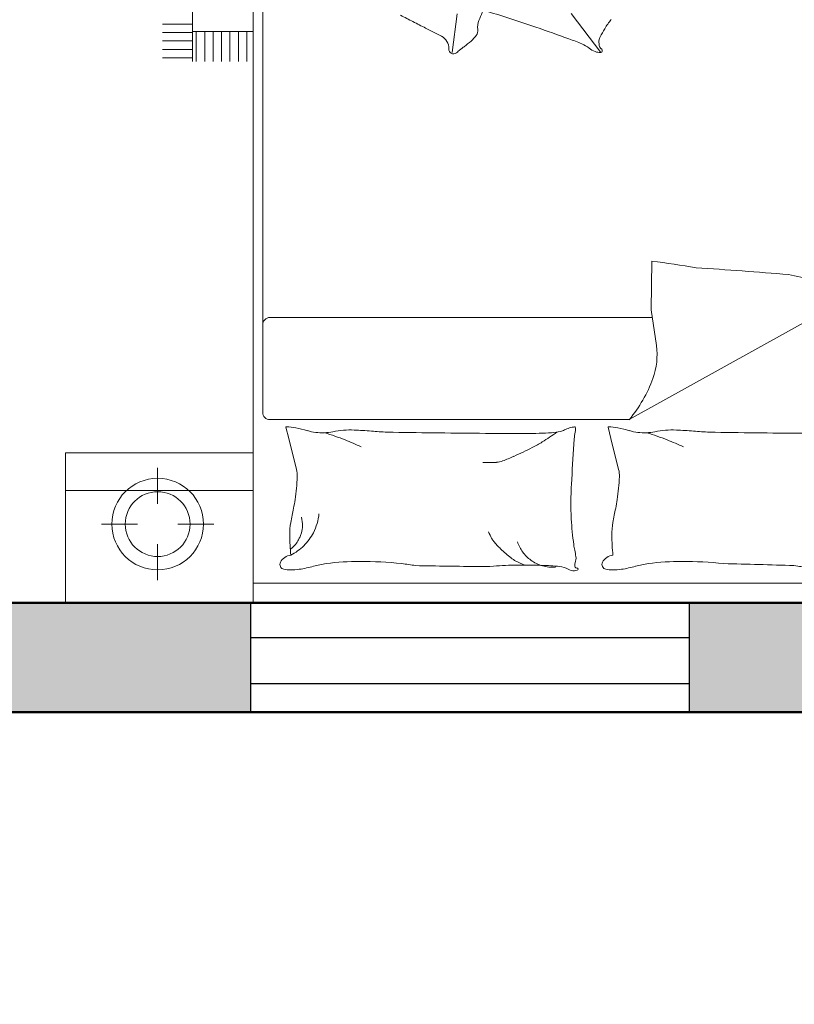
# Model space of a CAD drawing. Units: inches. Extents: x -7 to 1228, y -146 to 1091.
# Tile 36 of 88: x 1002 to 1066, y 36 to 117. Entities that reach past the tile are written whole.
import ezdxf

# ---------------------------------------------------------------- set-up
doc = ezdxf.new("R2010")
doc.units = ezdxf.units.IN
for name, color, linetype, lineweight in [('A-FURN', 8, 'Continuous', 18), ('A-GLAZ', 175, 'Continuous', 25), ('A-WALL', 7, 'Continuous', 50), ('A-WALL-PATT', 251, 'Continuous', 13)]:
    doc.layers.add(name, color=color, linetype=linetype, lineweight=lineweight)
doc.styles.add('DIM_FONT', font='SIMPLEX.shx', dxfattribs={"width": 0.8})

# ---------------------------------------------------------------- blocks, each defined once
blk = doc.blocks.new('A$C4F634EDD')
for p, q in [((0, 2.6295), (0, 2.2295)), ((0.5, 2.6295), (0, 2.6295)), ((0.5, 2.6295), (2.3, 2.6295)), ((0.5, 0.5295), (0.5, 2.6295)), ((0.5, 2.2295), (0.5, 2.6295)), ((0.5, 2.5771), (2.3, 2.5771)), ((0.2457, 2.5697), (0.2457, 2.4733)), ((0.0957, 2.4197), (0.192, 2.4197)), ((0.2994, 2.4197), (0.3957, 2.4197)), ((0.2457, 2.366), (0.2457, 2.2697)), ((0, 2.3301), (0.5, 2.3301)), ((0.5953, 2.1912), (0.616, 2.2738)), ((1.4546, 2.1912), (1.4752, 2.2738)), ((0, 2.2295), (0.5, 2.2295)), ((0.5878, 2.1612), (0.5953, 2.1912)), ((1.4471, 2.1612), (1.4546, 2.1912)), ((1.5035, 2.141), (0.5458, 2.141)), ((1.5035, 2.141), (2.2716, 1.7136)), ((0.5258, 2.121), (0.5258, 0.5617)), ((1.576, 1.9433), (1.5624, 1.8479)), ((0.5458, 1.8684), (1.5653, 1.8684)), ((1.5624, 1.8479), (1.5641, 1.7178)), ((0.3386, 0), (0.3386, 1.1852)), ((0.3486, 1.1052), (0.3486, 1.1852)), ((0.3711, 1.1052), (0.3711, 1.1852)), ((0.3936, 1.1052), (0.3936, 1.1852)), ((0.4161, 1.1052), (0.4161, 1.1852)), ((0.4386, 1.1052), (0.4386, 1.1852)), ((0.4611, 1.1052), (0.4611, 1.1852)), ((0.4836, 1.1052), (0.4836, 1.1852)), ((0.2586, 1.1753), (0.3386, 1.1753)), ((1.031, 1.1612), (1.0448, 1.0581)), ((1.4276, 1.1611), (1.3484, 1.0571)), ((0.2586, 1.1528), (0.3386, 1.1528)), ((0.2586, 1.1303), (0.3386, 1.1303)), ((0.2586, 1.1078), (0.3386, 1.1078)), ((0.3386, 1.1052), (0.5, 1.1052)), ((0.2586, 1.0853), (0.3386, 1.0853))]:
    blk.add_line(p, q)
for radius in [0.1222, 0.0865]:
    blk.add_circle((0.2457, 2.4197), radius)
for centre, radius, start, end in [((0.5848, 2.5274), 0.0131, 101.2724, 206.5805), ((0.5999, 2.4516), 0.0904, 90, 101.2724), ((0.5999, 2.3808), 0.1611, 81.5628, 90), ((0.5788, 2.2388), 0.3048, 74.256, 81.5628), ((0.7272, 2.7653), 0.2422, 254.256, 262.4531), ((0.7851, 3.2019), 0.6827, 262.4531, 270), ((0.7851, 3.5682), 1.049, 270, 276.0867), ((0.8402, 3.0514), 0.5293, 276.0867, 280.1899), ((1.1602, -8.1346), 10.6675, 90.30153, 91.21582), ((1.1169, 2.2433), 0.2897, 85.1982, 92.5386), ((1.2142, 3.4021), 0.8732, 265.1982, 269.4243), ((1.3082, 2.3102), 0.234, 110.8603, 117.2396), ((1.2204, 4.0232), 1.4943, 269.4243, 271.9079), ((1.2995, 2.4357), 0.0992, 105.9352, 126.0864), ((1.2429, 3.3501), 0.8208, 271.9079, 275.2592), ((1.2995, 2.4357), 0.0992, 85.7841, 105.9352), ((1.3132, 2.5864), 0.0539, 275.2592, 300.6513), ((1.3554, 2.5152), 0.0289, 85.6975, 120.6513), ((1.3556, 2.519), 0.0251, 68.2117, 85.6975), ((1.3739, 2.5288), 0.0156, 158.0096, 201.421), ((1.3634, 2.533), 0.00428, 78.1069, 158.0096), ((1.3288, 2.5111), 0.0328, 351.8665, 21.421), ((1.3647, 2.5395), 0.00232, 258.1069, 19.564), ((1.3637, 2.5391), 0.00342, 19.564, 68.2117), ((1.444, 2.5274), 0.0131, 101.2724, 206.5805), ((1.4591, 2.4516), 0.0904, 90, 101.2724), ((1.4591, 2.3808), 0.1611, 81.5628, 90), ((1.438, 2.2388), 0.3048, 74.256, 81.5628), ((1.5865, 2.7653), 0.2422, 254.256, 262.4531), ((1.6443, 3.2019), 0.6827, 262.4531, 270), ((1.6443, 3.5682), 1.049, 270, 276.0867), ((1.4785, 15.4878), 12.9656, 271.22425, 272.05324), ((1.97, 2.3805), 0.1524, 92.5386, 100.1899), ((0.6036, 2.5368), 0.0342, 206.5805, 265.5998), ((1.0898, 2.4496), 0.4918, 173.7676, 180), ((0.5368, 2.3783), 0.1399, 45.0976, 62.7964), ((1.4317, 2.2032), 0.3916, 128.3886, 133.8115), ((1.2362, 2.45), 0.0768, 117.2396, 128.3886), ((1.2995, 2.4357), 0.0992, 126.0864, 143.8234), ((1.1177, 2.5413), 0.246, 347.8905, 351.8665), ((1.4628, 2.5368), 0.0342, 206.5805, 265.5998), ((1.949, 2.4496), 0.4918, 173.7676, 180), ((0.5462, 2.4142), 0.0899, 41.4429, 53.7359), ((0.5741, 2.4389), 0.0526, 25.3551, 41.4429), ((0.5368, 2.3783), 0.1399, 27.3988, 45.0976), ((1.3165, 2.3233), 0.2252, 133.8115, 140.9651), ((1.2995, 2.4357), 0.0992, 143.8234, 161.5603), ((2.2605, 2.3525), 0.9131, 172.3191, 176.6313), ((1.5522, 2.448), 0.1983, 167.8905, 172.3191), ((0.8019, 2.4496), 0.204, 180, 189.6844), ((0.4851, 2.3967), 0.1511, 21.8149, 25.3551), ((0.4345, 2.3765), 0.2056, 18.7799, 21.8149), ((1.3127, 2.3625), 0.2002, 151.6832, 156.9972), ((1.1799, 2.4341), 0.0493, 140.9651, 151.6832), ((1.6611, 2.4496), 0.204, 180, 189.6844), ((0.576, 2.4246), 0.0562, 0, 18.7799), ((0.5406, 2.4246), 0.0915, 345.3149, 0), ((0.5368, 2.3783), 0.1399, 16.515, 27.3988), ((0.5368, 2.3783), 0.1399, 5.6311, 16.515), ((1.4703, 2.5637), 0.882, 189.6844, 192.1984), ((2.0266, 2.3663), 0.6787, 176.6313, 181.6331), ((2.3295, 2.5637), 0.882, 189.6844, 192.1984), ((0.2982, 2.3103), 0.3171, 8.0051, 12.1984), ((1.1575, 2.3103), 0.3171, 8.0051, 12.1984), ((-0.0401, 2.2627), 0.6588, 2.6649, 8.0051), ((2.7128, 2.3859), 1.3652, 181.6331, 183.055), ((0.8191, 2.2627), 0.6588, 2.6649, 8.0051), ((14.9657, 3.0398), 13.6356, 183.05496, 183.50486), ((0.5503, 2.2902), 0.0677, 345.9548, 2.6649), ((1.4096, 2.2902), 0.0677, 345.9548, 2.6649), ((1.1303, 1.9835), 0.2721, 85.9172, 93.5552), ((1.1455, 2.197), 0.058, 69.3257, 85.9172), ((0.9871, 1.7772), 0.5066, 65.6735, 69.3257), ((0.6058, 0.9338), 1.4323, 63.5015, 65.6735), ((0.473, 2.8815), 0.7387, 293.4844, 295.3111), ((1.1054, 1.9358), 0.3126, 57.865, 63.5015), ((1.3322, 2.8815), 0.7387, 293.4844, 295.3111), ((0.473, 2.8815), 0.7387, 287.1982, 289.428), ((0.473, 2.8815), 0.7387, 289.428, 291.6577), ((0.473, 2.8815), 0.7387, 291.6577, 293.4844), ((0.8841, 1.5835), 0.7286, 54.1737, 57.865), ((1.6762, 2.2258), 0.3212, 183.5049, 189.9984), ((1.3322, 2.8815), 0.7387, 287.1982, 289.428), ((1.3322, 2.8815), 0.7387, 289.428, 291.6577), ((1.3322, 2.8815), 0.7387, 291.6577, 293.4844), ((0.5887, 2.1609), 0.000917, 165.9551, 274.0829), ((0.5695, 2.4301), 0.2708, 274.0829, 279.4841), ((0.5763, 2.3896), 0.2297, 279.4841, 287.3864), ((0.6807, 2.0561), 0.1197, 96.4341, 107.3864), ((0.6836, 2.0301), 0.1459, 78.4414, 96.4341), ((0.759, 2.3985), 0.2301, 258.4414, 272.7491), ((0.7026, 3.5718), 1.4048, 272.7491, 274.6176), ((0.9136, 0.9591), 1.2165, 92.6096, 94.6176), ((1.2501, -19.8405), 22.0183, 90.37908, 91.01965), ((1.2012, -3.5404), 5.7185, 89.7135, 90.9704), ((1.224, 1.0141), 1.164, 86.426, 89.7135), ((1.2875, 2.0302), 0.1459, 77.131, 86.426), ((1.3099, 2.1283), 0.0453, 62.7159, 77.131), ((1.3658, 2.2367), 0.0767, 242.7159, 253.7788), ((1.3688, 2.247), 0.0875, 253.7788, 262.8796), ((1.3581, 2.1615), 0.00132, 262.8796, 343.3022), ((1.3409, 2.1667), 0.0193, 343.3022, 9.9984), ((1.448, 2.1609), 0.000917, 165.9551, 274.0829), ((1.4288, 2.4301), 0.2708, 274.0829, 279.4841), ((1.4355, 2.3896), 0.2297, 279.4841, 287.3864), ((1.5399, 2.0561), 0.1197, 96.4341, 107.3864), ((1.5429, 2.0301), 0.1459, 78.4414, 96.4341), ((1.6182, 2.3985), 0.2301, 258.4414, 272.7491), ((1.5619, 3.5718), 1.4048, 272.7491, 274.6176), ((1.7729, 0.9591), 1.2165, 92.6096, 94.6176), ((2.1093, -19.8405), 22.0183, 90.37908, 91.01965), ((0.5458, 2.121), 0.02, 90, 180), ((1.2147, 1.9017), 0.3751, 20.1488, 39.6445), ((1.3977, 1.9688), 0.1801, 351.8644, 20.1488), ((0.5458, 1.8884), 0.02, 180, 270), ((1.4194, 4.2174), 2.5158, 281.6741, 283.1904), ((1.0582, 5.4638), 3.7801, 277.692, 279.495), ((0.6102, 18.0525), 16.3521, 273.75703, 274.62393), ((1.0348, 1.1521), 0.0127, 51.1864, 183.2455), ((0.9991, 1.1077), 0.0697, 45.8726, 51.1864), ((1.0791, 1.1902), 0.0452, 225.8726, 232.4713), ((1.4338, 1.1026), 0.0601, 110.3452, 128.5854), ((1.4251, 1.1259), 0.0352, 86.0516, 110.3452), ((1.4273, 1.1567), 0.00443, 13.2808, 86.0516), ((1.4254, 1.1562), 0.0063, 306.5792, 13.2808), ((0.9863, 1.1494), 0.0359, 297.2902, 3.2455), ((1.2846, 1.4577), 0.3825, 232.4713, 233.7837), ((0.6683, 0.6162), 0.6605, 52.7849, 53.7837), ((0.9362, 0.9689), 0.2176, 46.4776, 52.7849), ((1.0543, 1.9106), 0.8371, 290.1287, 292.7069), ((1.3469, 1.2115), 0.0792, 292.7069, 308.5854), ((1.4996, 1.1284), 0.0771, 169.5926, 177.2714), ((1.4378, 1.1314), 0.0153, 177.2714, 194.5709), ((1.4376, 1.1398), 0.0142, 126.5792, 169.5926), ((-0.4173, 3.8699), 3.0972, 296.4147, 297.2902), ((1.0327, 1.0706), 0.0774, 35.8936, 46.4776), ((1.0771, 1.1027), 0.0226, 351.9508, 35.8936), ((-0.4107, 5.9078), 5.0942, 289.0836, 290.1287), ((1.4611, 1.1374), 0.0393, 194.5709, 206.8179), ((1.7401, 1.2785), 0.352, 206.8179, 210.9056), ((3.744, -4.3336), 6.1019, 117.49986, 117.84822), ((1.8575, -0.7096), 2.0162, 116.4147, 117.4999), ((1.1449, 1.0931), 0.0458, 171.9508, 202.4162), ((0.2266, 4.0657), 3.145, 286.6085, 289.0836), ((1.6045, 1.1973), 0.194, 210.9056, 219.7005), ((2.032, 1.4591), 1.0054, 202.4162, 205.0529)]:
    blk.add_arc(centre, radius, start, end)
at = {"style": 'DIM_FONT', "width": 0.8, "flags": 9}
for tag, p in [('YSIZE', (0.5, 2.6295)), ('XSIZE', (0.5, 2.6295)), ('XSIZE', (2.2985, 2.6295)), ('YSIZE', (2.2985, 2.6295))]:
    blk.add_attdef(tag, p, '', height=0.0005, dxfattribs=at)
blk = doc.blocks.new('WIN-36')
for p, q in [((0, 36), (0, 0)), ((9, 36), (0, 36)), ((2.343, 36), (2.343, 0)), ((6.137, 0), (6.137, 36)), ((9, 0), (9, 36)), ((0, 0), (9, 0)), ((2.343, 0), (6.137, 0))]:
    blk.add_line(p, q)

msp = doc.modelspace()

# ---------------------------------------------------------------- hatches: boundary and pattern name
at = {"layer": 'A-WALL-PATT'}
h = msp.add_hatch(color=256, dxfattribs=at)
h.dxf.hatch_style = 1
h.paths.add_polyline_path([(69, 568), (60, 568), (60, 493), (63.289, 493), (69, 493)])
h.paths.add_polyline_path([(69, 662.405), (60, 662.405), (60, 586), (69, 586)], flags=17)
h.paths.add_polyline_path([(69, 723), (184, 723), (184, 734), (179, 734), (179, 728), (69, 728), (69, 741.623), (60, 741.623), (60, 698.405), (69, 698.405)], flags=17)
h.paths.add_polyline_path([(69, 782), (231, 782), (231, 728), (231, 723), (231, 586), (236, 586), (236, 787), (69, 787), (69, 800.126), (60, 800.126), (60, 765.623), (69, 765.623)])
h.paths.add_polyline_path([(184, 842), (189, 842), (189, 848), (173, 848), (173, 842), (179, 842), (179, 787), (184, 787)])
h.paths.add_polyline_path([(118.22, 69), (69, 69), (69, 60), (118.22, 60)])
h.paths.add_polyline_path([(227, 69), (154.22, 69), (154.22, 60), (227, 60)])
h.paths.add_polyline_path([(236, 60), (232.711, 60), (227, 60), (227, 36), (236, 36)])
h.paths.add_polyline_path([(389, 60), (380, 60), (380, 36), (389, 36)])
h.paths.add_polyline_path([(384, 181), (380, 181), (380, 115), (380, 78), (384, 78)])
h.paths.add_polyline_path([(380, 115), (334.547, 115), (334.547, 109), (380, 109)])
h.paths.add_polyline_path([(274.547, 115), (236, 115), (236, 201), (232.711, 201), (231, 201), (231, 78), (236, 78), (236, 109), (274.547, 109)])
h.paths.add_polyline_path([(69, 123), (60, 123), (60, 78), (69, 78)])
h.paths.add_polyline_path([(69, 201), (60, 201), (60, 159), (69, 159)])
h.paths.add_polyline_path([(143, 219), (69, 219), (69, 213), (143, 213)], flags=17)
h.paths.add_polyline_path([(189, 219), (184, 219), (184, 274), (231, 274), (231, 219), (236, 219), (236, 279), (184, 279), (184, 297), (179, 297), (179, 279), (69, 279), (69, 290.912), (60, 290.912), (60, 262.179), (69, 262.179), (69, 274), (179, 274), (179, 219), (173, 219), (173, 213), (189, 213)])
h.paths.add_polyline_path([(69, 238.179), (60, 238.179), (60, 219), (69, 219)], flags=17)
h.paths.add_polyline_path([(69, 333), (60, 333), (60, 314.912), (69, 314.912), (69, 316.965)])
h.paths.add_polyline_path([(190, 338), (184, 338), (69, 338), (69, 333), (179, 333), (179, 327), (184, 327), (184, 333.021), (190, 333.046)])
h.paths.add_polyline_path([(69, 386.806), (60, 386.806), (60, 351), (69, 351)])
h.paths.add_polyline_path([(69, 475), (60, 475), (60, 422.806), (69, 422.806)])
h.paths.add_polyline_path([(236, 475), (231, 475), (231, 351.238), (236, 351.238)])
h.paths.add_polyline_path([(384, 475), (380, 475), (380, 362), (384, 362)])
h.paths.add_polyline_path([(547, 307), (439, 307), (439, 356), (445, 356), (445, 362), (433, 362), (433, 307), (380, 307), (380, 244), (380, 241), (384, 241), (384, 301), (433, 301), (433, 277), (439, 277), (439, 301), (547, 301)])
h.paths.add_polyline_path([(547, 241), (439, 241), (439, 247), (433, 247), (433, 235), (547, 235)])
h.paths.add_polyline_path([(450, 69), (440.286, 69), (424.889, 69), (389, 69), (389, 60), (450, 60)])
h.paths.add_polyline_path([(547, 69), (486, 69), (486, 60), (547, 60)])
h.paths.add_polyline_path([(556, 148.268), (547, 148.268), (547, 78), (556, 78)])
h.paths.add_polyline_path([(556, 223), (547, 223), (547, 195), (547, 184.268), (556, 184.268)])
h.paths.add_polyline_path([(556, 311.192), (547, 311.192), (547, 273.075), (556, 273.075)])
h.paths.add_polyline_path([(556, 344), (552.711, 344), (547, 344), (547, 335.192), (556, 335.192)])
h.paths.add_polyline_path([(556, 249.075), (547, 249.075), (547, 241), (556, 241)])
h.paths.add_polyline_path([(547, 362), (475, 362), (475, 356), (547, 356)], flags=0)
h.paths.add_polyline_path([(556, 399.621), (547, 399.621), (547, 362), (556, 362)])
h.paths.add_polyline_path([(556, 475), (547, 475), (547, 435.621), (556, 435.621)])
h.paths.add_polyline_path([(547, 493), (389, 493), (389, 487), (547, 487)])
h.paths.add_polyline_path([(380, 493), (278, 493), (278, 487), (380, 487)])
h.paths.add_polyline_path([(227, 493), (69, 493), (69, 487), (227, 487)])
h.paths.add_polyline_path([(643, 122.445), (634, 122.445), (634, 78), (643, 78)])
h.paths.add_polyline_path([(702.5, 69), (692.786, 69), (677.389, 69), (643, 69), (643, 60), (702.5, 60)])
h.paths.add_polyline_path([(798, 69), (738.5, 69), (738.5, 60), (798, 60)])
h.paths.add_polyline_path([(807, 60), (803.711, 60), (798, 60), (798, 36), (807, 36)])
h.paths.add_polyline_path([(807, 109), (846.751, 109), (846.751, 115), (807, 115), (807, 159), (802, 159), (802, 78), (807, 78)])
h.paths.add_polyline_path([(807, 201), (802, 201), (802, 195), (807, 195)])
h.paths.add_polyline_path([(643, 201), (634, 201), (634, 158.445), (643, 158.445)])
h.paths.add_polyline_path([(756, 225), (751, 225), (751, 219), (643, 219), (643, 213), (756, 213)])
h.paths.add_polyline_path([(643, 240.848), (634, 240.848), (634, 219), (643, 219)])
h.paths.add_polyline_path([(643, 274), (643, 288.629), (634, 288.629), (634, 264.848), (643, 264.848)])
h.paths.add_polyline_path([(802, 279), (756, 279), (756, 297), (751, 297), (751, 279), (643, 279), (643, 274), (751, 274), (751, 255), (756, 255), (756, 274), (802, 274)])
h.paths.add_polyline_path([(807, 333), (803.711, 333), (802, 333), (802, 279), (802, 274), (802, 219), (807, 219)])
h.paths.add_polyline_path([(956, 182), (951, 182), (951, 115), (906.751, 115), (906.751, 109), (951, 109), (951, 78), (956, 78)])
h.paths.add_polyline_path([(960, 60), (951, 60), (951, 36), (960, 36)])
h.paths.add_polyline_path([(1021, 69), (1005.781, 69), (960, 69), (960, 60), (1021, 60)])
h.paths.add_polyline_path([(956, 224), (951, 224), (951, 218), (956, 218)])
h.paths.add_polyline_path([(956, 302), (1004, 302), (1004, 278), (1010, 278), (1010, 302), (1118, 302), (1118, 290.809), (1127, 290.809), (1127, 326.968), (1118, 326.968), (1118, 320.966), (1118, 307), (1010, 307), (1010, 356), (1016, 356), (1016, 362), (1004, 362), (1004, 307), (951, 307), (951, 244), (951, 242), (954.289, 242), (956, 242)])
h.paths.add_polyline_path([(643, 333), (634, 333), (634, 312.629), (643, 312.629), (643, 316.965)])
h.paths.add_polyline_path([(756, 338), (643, 338), (643, 333), (751, 333), (751, 327), (756, 327)])
h.paths.add_polyline_path([(643, 388), (634, 388), (634, 351), (643, 351)])
h.paths.add_polyline_path([(807, 357), (802, 357), (802, 351), (807, 351)])
h.paths.add_polyline_path([(807, 475), (802, 475), (802, 393), (807, 393)])
h.paths.add_polyline_path([(643, 475), (634, 475), (634, 424), (643, 424)])
h.paths.add_polyline_path([(798, 493), (643, 493), (643, 487), (798, 487)])
h.paths.add_polyline_path([(634, 493), (556, 493), (556, 487), (634, 487)])
h.paths.add_polyline_path([(813, 493), (807, 493), (807, 487), (813, 487)])
h.paths.add_polyline_path([(951, 493), (849, 493), (849, 487), (951, 487)])
h.paths.add_polyline_path([(956, 484), (951, 484), (951, 374), (956, 374)])
h.paths.add_polyline_path([(1109, 493), (969, 493), (969, 487), (1109, 487)])
h.paths.add_polyline_path([(1127, 484), (1118, 484), (1118, 450.641), (1127, 450.641)])
h.paths.add_polyline_path([(1127, 414.641), (1118, 414.641), (1118, 365), (1127, 365)])
h.paths.add_polyline_path([(1109, 362), (1046, 362), (1046, 356), (1109, 356)], flags=17)
h.paths.add_polyline_path([(1127, 356), (1123.454, 356), (1118, 356), (1118, 350.968), (1127, 350.968)], flags=0)
h.paths.add_polyline_path([(1127, 266.809), (1118, 266.809), (1118, 262.361), (1118, 242), (1127, 242)], flags=17)
h.paths.add_polyline_path([(1118, 242), (1010, 242), (1010, 248), (1004, 248), (1004, 237), (1118, 237)])
h.paths.add_polyline_path([(1127, 224), (1118, 224), (1118, 170), (1127, 170)])
h.paths.add_polyline_path([(1127, 134), (1118, 134), (1118, 78), (1127, 78)])
h.paths.add_polyline_path([(1118, 69), (1057, 69), (1057, 60), (1118, 60)])
h.paths.add_polyline_path([(227, 571.546), (227, 574), (69, 574), (69, 568), (227, 568)])
h.paths.add_polyline_path([(380, 571.546), (380, 574), (278, 574), (278, 568), (380, 568)])
h.paths.add_polyline_path([(242, 574), (236, 574), (236, 568), (242, 568)])
h.paths.add_polyline_path([(547, 571.546), (547, 574), (389, 574), (389, 568), (547, 568)])
h.paths.add_polyline_path([(384, 733), (380, 733), (380, 586), (384, 586)])
h.paths.add_polyline_path([(556, 646), (634, 646), (634, 655), (547, 655), (547, 586), (556, 586)])
h.paths.add_polyline_path([(634, 574), (556, 574), (556, 568), (634, 568)])
h.paths.add_polyline_path([(643, 655), (634, 655), (634, 586), (643, 586)])
h.paths.add_polyline_path([(798, 574), (643, 574), (643, 568), (798, 568)])
h.paths.add_polyline_path([(643, 663.854), (634, 663.854), (634, 655), (643, 655)])
h.paths.add_polyline_path([(556, 676.967), (547, 676.967), (547, 655), (556, 655)])
h.paths.add_polyline_path([(556, 733), (547, 733), (547, 712.967), (556, 712.967)])
h.paths.add_polyline_path([(643, 710), (634, 710), (634, 699.854), (643, 699.854)])
h.paths.add_polyline_path([(807, 668), (802, 668), (802, 586), (807, 586)])
h.paths.add_polyline_path([(951, 574), (849, 574), (849, 568), (951, 568)])
h.paths.add_polyline_path([(956, 691), (951, 691), (951, 577), (956, 577)])
h.paths.add_polyline_path([(1109, 574), (969, 574), (969, 568), (1109, 568)])
h.paths.add_polyline_path([(1127, 643.403), (1118, 643.403), (1118, 577), (1127, 577)])
h.paths.add_polyline_path([(1127, 568), (1123.454, 568), (1118, 568), (1118, 493), (1127, 493)])
h.paths.add_polyline_path([(1127, 733), (1118, 733), (1118, 679.403), (1127, 679.403)])
h.paths.add_polyline_path([(1127, 777.348), (1118, 777.348), (1118, 770.035), (1118, 751), (1127, 751)], flags=17)
h.paths.add_polyline_path([(1118, 751), (1010, 751), (1010, 757), (1004, 757), (1004, 745), (1118, 745)])
h.paths.add_polyline_path([(956, 811), (1004, 811), (1004, 787), (1010, 787), (1010, 811), (1017.874, 811), (1017.874, 811.627, -0.414214), (1018.247, 812), (1031.978, 812, -0.414214), (1032.351, 811.627), (1032.351, 811), (1118, 811), (1118, 801.348), (1127, 801.348), (1127, 834.685), (1118, 834.685), (1118, 830.238), (1118, 817), (1010, 817), (1010, 866), (1016, 866), (1016, 872), (1004, 872), (1004, 817), (956, 817), (956, 866), (951, 866), (951, 751), (954.289, 751), (956, 751)])
h.paths.add_polyline_path([(1118, 872), (1046, 872), (1046, 866), (1118, 866)], flags=17)
h.paths.add_polyline_path([(1127, 924.711), (1118, 924.711), (1118, 884), (1127, 884)])
h.paths.add_polyline_path([(1127, 866), (1123.711, 866), (1118, 866), (1118, 858.685), (1127, 858.685)], flags=17)
h.paths.add_polyline_path([(956, 983), (951, 983), (951, 952), (807, 952), (807, 983), (802, 983), (802, 902), (807, 902), (807, 946), (951, 946), (951, 884), (956, 884)])
h.paths.add_polyline_path([(807, 842), (802, 842), (802, 787), (756, 787), (756, 806), (751, 806), (751, 787), (643, 787), (643, 782), (751, 782), (751, 764), (756, 764), (756, 782), (802, 782), (802, 728), (807, 728)])
h.paths.add_polyline_path([(756, 848), (643, 848), (643, 842), (751, 842), (751, 836), (756, 836)])
h.paths.add_polyline_path([(756, 734), (751, 734), (751, 728), (643, 728), (643, 723), (756, 723)])
h.paths.add_polyline_path([(643, 749.791), (634, 749.791), (634, 728), (637.289, 728), (643, 728)])
h.paths.add_polyline_path([(643, 805.405), (634, 805.405), (634, 773.791), (643, 773.791)])
h.paths.add_polyline_path([(643, 896.663), (634, 896.663), (634, 860), (637.289, 860), (643, 860)])
h.paths.add_polyline_path([(643, 842), (634, 842), (634, 829.405), (643, 829.405)])
h.paths.add_polyline_path([(643, 983), (634, 983), (634, 932.663), (643, 932.663)])
h.paths.add_polyline_path([(1127, 983), (1118, 983), (1118, 960.711), (1127, 960.711)])
h.paths.add_polyline_path([(1118, 1001), (1077.525, 1001), (1077.525, 992), (1118, 992)])
h.paths.add_polyline_path([(1041.525, 1001), (960, 1001), (960, 992), (1041.525, 992)])
h.paths.add_polyline_path([(960, 1025), (951, 1025), (951, 1001), (954.289, 1001), (960, 1001)])
h.paths.add_polyline_path([(807, 1025), (798, 1025), (798, 1001), (807, 1001)])
h.paths.add_polyline_path([(798, 1001), (738.5, 1001), (738.5, 992), (798, 992)])
h.paths.add_polyline_path([(702.5, 1001), (643, 1001), (643, 992), (702.5, 992)])
h.paths.add_polyline_path([(547, 1001), (499.113, 1001), (499.113, 992), (547, 992)])
h.paths.add_polyline_path([(463.113, 1001), (389, 1001), (389, 992), (463.113, 992)])
h.paths.add_polyline_path([(389, 1025), (380, 1025), (380, 1022), (380, 1001), (383.289, 1001), (389, 1001)])
h.paths.add_polyline_path([(236, 1025), (227, 1025), (227, 1001), (236, 1001)])
h.paths.add_polyline_path([(236, 983), (231, 983), (231, 860), (236, 860)])
h.paths.add_polyline_path([(274.547, 952), (236, 952), (236, 946), (274.547, 946)])
h.paths.add_polyline_path([(380, 952), (334.547, 952), (334.547, 946), (380, 946)])
h.paths.add_polyline_path([(384, 983), (380, 983), (380, 884), (383.289, 884), (384, 884)])
h.paths.add_polyline_path([(227, 1001), (155.012, 1001), (155.012, 992), (162.875, 992), (227, 992)])
h.paths.add_polyline_path([(119.012, 1001), (69, 1001), (69, 992), (119.012, 992)])
h.paths.add_polyline_path([(69, 983), (60, 983), (60, 922.987), (69, 922.987)])
h.paths.add_polyline_path([(69, 886.987), (60, 886.987), (60, 860), (63.289, 860), (69, 860)])
h.paths.add_polyline_path([(143, 848), (69, 848), (69, 842), (143, 842)])

# ---------------------------------------------------------------- linework, layer by layer
at = {"layer": 'A-WALL'}
for p, q in [((1127, 69), (951, 69)), ((1127, 60), (951, 60)), ((951, 60), (1127, 60))]:
    msp.add_line(p, q, dxfattribs=at)

# ---------------------------------------------------------------- block references
at = {"layer": 'A-FURN', "xscale": -30.79356024027943, "yscale": 30.79356024027943, "zscale": 30.79356024027943, "rotation": 180}
msp.add_blockref('A$C4F634EDD', (1005.781, 149.972), dxfattribs=at)
at = {"layer": 'A-GLAZ', "extrusion": (0, 0, -1), "zscale": -1, "rotation": 90.00000000000007}
msp.add_blockref('WIN-36', (-1021, 60), dxfattribs=at)

doc.saveas('drawing.dxf')
